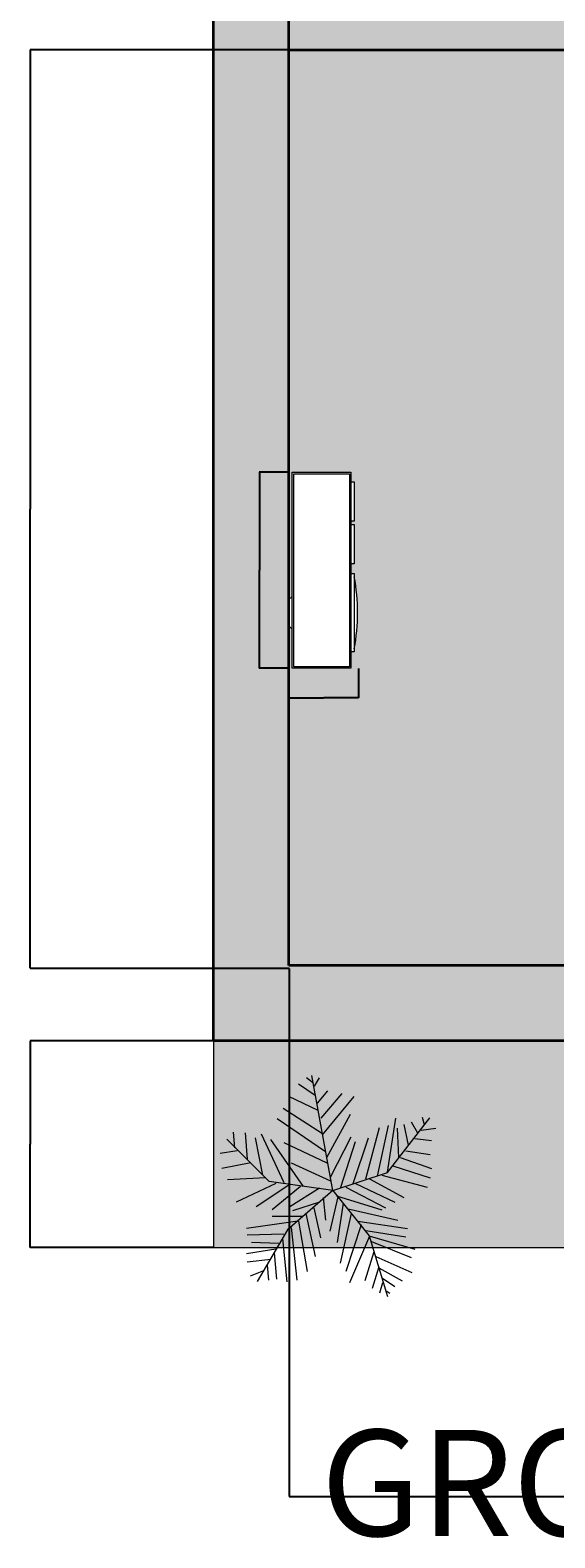
# Model space of a CAD drawing. Units: millimetres. Extents: x 1166 to 16630, y -7192 to 2820.
# Tile 1 of 8: x 1166 to 2769, y -7192 to -2583. Entities that reach past the tile are written whole.
import ezdxf

# ---------------------------------------------------------------- set-up
doc = ezdxf.new("R2010")
doc.units = ezdxf.units.MM
for name, color, linetype, lineweight in [('A-ANNO-DIMS', 2, 'Continuous', 18), ('A-ANNO-TEXT', 7, 'Continuous', 35), ('A-FURN', 8, 'Continuous', 18), ('A-WALL', 7, 'Continuous', 35), ('C-SITE-PAVE', 7, 'Continuous', 18), ('L-PLNT', 70, 'Continuous', 18), ('L-PLNT-PATT', 3, 'Continuous', 13)]:
    doc.layers.add(name, color=color, linetype=linetype, lineweight=lineweight)
doc.layers.add('A-FLOR-FNSH-PATT', color=254, linetype='Continuous', lineweight=13, true_color=0xfeeab9)
doc.layers.add('A-WALL-PATT', color=254, linetype='Continuous', lineweight=13, true_color=0xcecce6)
doc.styles.get("Standard").update_dxf_attribs({"font": 'arial.ttf'})
doc.dimstyles.get("Standard").update_dxf_attribs({"dimtxt": 0.18, "dimasz": 0.18, "dimexe": 0.18, "dimexo": 0.0625, "dimgap": 0.09, "dimtad": 0, "dimtih": 1, "dimtoh": 1, "dimdec": 4, "dimzin": 0, "dimdsep": 46, "dimtxsty": 'Standard', "dimcen": 0.09, "dimadec": 0, "dimazin": 0, "dimtfac": 1, "dimtdec": 4, "dimtofl": 0, "dimtmove": 0, "dimatfit": 3, "dimfxl": 1, "dimtolj": 1, "dimtzin": 0, "dimarcsym": 0})

# ---------------------------------------------------------------- blocks, each defined once
blk = doc.blocks.new('Entertainment Center')
for p, q in [((-4, 0), (-5, -1)), ((4, 0), (-4, 0)), ((5, -1), (4, 0)), ((-17, -19), (-17, -1)), ((-17, -1), (43, -1)), ((-16.5, -18.5), (-16.5, -1.5)), ((-16.5, -1.5), (42.5, -1.5)), ((42.5, -1.5), (42.5, -18.5)), ((43, -1), (43, -19)), ((43, -19), (-17, -19)), ((42.5, -18.5), (-16.5, -18.5)), ((-12, -20), (-12, -19)), ((12, -20), (-12, -20)), ((12, -19), (12, -20)), ((15, -20), (15, -19)), ((27, -20), (15, -20)), ((27, -19), (27, -20)), ((28, -20), (28, -19)), ((40, -20), (28, -20)), ((40, -19), (40, -20))]:
    blk.add_line(p, q)
blk.add_arc((0, 40), 61, 259.6111, 280.3889)
blk = doc.blocks.new('*U12')
for p, q in [((-8.737, 47.138), (-17.069, 52.711)), ((-10.186, 53.64), (-13.084, 55.962)), ((0, 0), (-10.5, 57)), ((-9.099, 51.782), (-6.563, 55.962)), ((-7.288, 39.707), (-21.778, 46.673)), ((-7.65, 43.423), (-2.578, 49.46)), ((-5.839, 35.992), (4.667, 48.067)), ((-5.114, 27.632), (10.463, 46.673)), ((-5.114, 28.097), (-24.676, 40.636)), ((-2.941, 16.486), (8.652, 37.85)), ((-3.665, 19.273), (-27.574, 35.527)), ((16.259, 5.805), (23.142, 31.348)), ((22.055, 7.198), (27.489, 32.277)), ((27, 9), (48, 36)), ((27.127, 9.056), (31.112, 35.992)), ((31.836, 30.883), (32.561, 16.486)), ((35.096, 32.741), (37.27, 22.524)), ((38.719, 34.134), (41.979, 28.561)), ((43.791, 29.954), (51.036, 30.883)), ((44.153, 36.456), (45.239, 32.741)), ((-31.5, 4.5), (-52.5, 25.5)), ((-48.585, 21.131), (-49.309, 29.026)), ((-43.513, 28.561), (-42.427, 15.558)), ((-38.442, 26.239), (-34.819, 7.663)), ((-35.544, 28.097), (-24.314, 3.947)), ((-14.533, 2.09), (-30.834, 25.31)), ((-24.314, 23.917), (-2.941, 13.7)), ((-1.129, 6.734), (9.014, 26.704)), ((3.942, 1.625), (11.187, 24.381)), ((10.101, 3.483), (17.708, 26.239)), ((40.53, 25.775), (48.862, 24.846)), ((-47.498, 19.737), (-55.83, 18.344)), ((33.285, 16.486), (48.862, 10.913)), ((36.183, 19.737), (48.137, 17.88)), ((-40.615, 13.7), (-55.105, 10.913)), ((-20.691, 13.7), (-1.129, 4.876)), ((0, 0), (27, 9)), ((24.229, 7.663), (46.688, 1.625)), ((29.662, 12.307), (48.137, 6.269)), ((-33.37, 6.269), (-52.207, 5.34)), ((-28.299, 3.483), (-47.86, -5.805)), ((-21.416, 3.018), (-38.079, -8.128)), ((0, 0), (-31.5, 4.5)), ((-15.982, 2.09), (-30.11, -9.521)), ((0, 0), (-22.5, -19.5)), ((-6.563, 1.161), (-21.416, -8.128)), ((0, 0), (18, -22.5)), ((6.478, 1.625), (26.04, -8.592)), ((11.187, 3.483), (30.749, -5.805)), ((18.07, 5.805), (35.096, -3.483)), ((-6.563, -5.805), (-19.967, -9.985)), ((-4.752, -3.483), (-3.665, -14.629)), ((2.493, -3.019), (-1.491, -20.202)), ((1.769, -2.555), (24.229, -9.521)), ((5.029, -6.27), (2.131, -25.775)), ((-15.257, -12.772), (-30.11, -12.772)), ((-13.446, -11.378), (-8.737, -32.741)), ((-9.461, -8.592), (-6.201, -23.453)), ((9.014, -11.378), (3.58, -35.992)), ((7.565, -9.056), (32.198, -14.629)), ((-17.431, -15.094), (-42.789, -18.809)), ((-24.314, -21.596), (-42.427, -22.06)), ((-22.5, -19.5), (-37.5, -45)), ((-20.691, -18.345), (-17.793, -44.352)), ((-17.069, -15.094), (-12.721, -40.172)), ((14.085, -16.951), (6.478, -40.172)), ((12.274, -15.094), (36.907, -18.809)), ((16.259, -19.738), (36.183, -22.989)), ((-28.299, -29.026), (-42.789, -31.348)), ((-26.849, -26.24), (-40.253, -25.775)), ((-25.038, -23.918), (-22.865, -45.281)), ((18.07, -22.524), (8.289, -45.745)), ((18, -22.5), (27, -52.5)), ((18.433, -22.524), (40.53, -29.026)), ((19.157, -25.311), (38.719, -33.206)), ((-30.834, -34.135), (-42.427, -35.528)), ((-32.646, -36.921), (-31.921, -44.352)), ((-29.023, -30.884), (-27.936, -43.887)), ((20.244, -30.419), (15.897, -44.816)), ((21.331, -32.741), (39.081, -40.636)), ((-34.457, -39.708), (-40.978, -42.494)), ((22.78, -37.85), (19.519, -48.532)), ((22.78, -38.314), (34.372, -44.816)), ((24.591, -43.423), (30.749, -47.603)), ((24.591, -45.745), (23.142, -50.854)), ((26.764, -49.925), (28.213, -50.854))]:
    blk.add_line(p, q)
blk = doc.blocks.new('*D17')
at = {"layer": 'A-ANNO-DIMS', "color": 0, "lineweight": -2, "transparency": 16777216}
for p, q in [((1955.9, -3933.8), (1865.8, -3933.8)), ((1866, -3934), (1866, -4233.5)), ((1866, -4533.4), (1866, -4233.8)), ((1955.9, -4533.5), (1865.8, -4533.5))]:
    blk.add_line(p, q, dxfattribs=at)
at = {"layer": 'A-ANNO-DIMS', "color": 0, "transparency": 16777216}
for points in [[(1865.9, -3934), (1866, -3934), (1866, -3933.8)], [(1865.9, -4533.4), (1866, -4533.4), (1866, -4533.5)]]:
    blk.add_solid(points, dxfattribs=at)
at = {"layer": 'Defpoints', "color": 0, "transparency": 16777216}
for p in [(1866, -3933.8), (1955.9, -3933.8), (1955.9, -4533.5)]:
    blk.add_point(p, dxfattribs=at)
at = {"layer": 'A-ANNO-DIMS', "color": 0, "transparency": 16777216, "insert": (1866, -4233.7), "char_height": 0.18, "attachment_point": 5}
blk.add_mtext('\\A1;TV UNIT 600 TYP.', dxfattribs=at)
blk = doc.blocks.new('*D18')
at = {"layer": 'A-ANNO-DIMS', "color": 0, "lineweight": -2, "transparency": 16777216}
for p, q in [((1955.9, -4533.6), (1955.9, -4623.7)), ((2169.2, -4533.6), (2169.2, -4623.7)), ((1956.1, -4623.5), (2062, -4623.5)), ((2169, -4623.5), (2063.2, -4623.5))]:
    blk.add_line(p, q, dxfattribs=at)
at = {"layer": 'A-ANNO-DIMS', "color": 0, "transparency": 16777216}
for points in [[(1956.1, -4623.5), (1956.1, -4623.5), (1955.9, -4623.5)], [(2169, -4623.5), (2169, -4623.5), (2169.2, -4623.5)]]:
    blk.add_solid(points, dxfattribs=at)
at = {"layer": 'Defpoints', "color": 0, "transparency": 16777216}
for p in [(1955.9, -4533.5), (2169.2, -4533.5), (1955.9, -4623.5)]:
    blk.add_point(p, dxfattribs=at)
at = {"layer": 'A-ANNO-DIMS', "color": 0, "transparency": 16777216, "insert": (2062.6, -4623.5), "char_height": 0.18, "attachment_point": 5}
blk.add_mtext('\\A1;213 TYP.', dxfattribs=at)
blk = doc.blocks.new('*D30')
at = {"layer": 'A-ANNO-DIMS', "color": 0, "lineweight": -2, "transparency": 16777216}
for p, q in [((1955.9, -2642.5), (1165.9, -2642.5)), ((1166.1, -2642.7), (1166.1, -4046.5)), ((1166.1, -5450.7), (1166.1, -4046.9)), ((1956.9, -5450.8), (1165.9, -5450.8))]:
    blk.add_line(p, q, dxfattribs=at)
at = {"layer": 'A-ANNO-DIMS', "color": 0, "transparency": 16777216}
for points in [[(1166.1, -2642.7), (1166.1, -2642.7), (1166.1, -2642.5)], [(1166.1, -5450.7), (1166.1, -5450.7), (1166.1, -5450.8)]]:
    blk.add_solid(points, dxfattribs=at)
at = {"layer": 'Defpoints', "color": 0, "transparency": 16777216}
for p in [(1955.9, -2642.5), (1166.1, -5450.8), (1957, -5450.8)]:
    blk.add_point(p, dxfattribs=at)
at = {"layer": 'A-ANNO-DIMS', "color": 0, "transparency": 16777216, "insert": (1166.1, -4046.7), "char_height": 0.18, "attachment_point": 5}
blk.add_mtext('\\A1;2808.3', dxfattribs=at)
blk = doc.blocks.new('*D31')
at = {"layer": 'A-ANNO-DIMS', "color": 0, "lineweight": -2, "transparency": 16777216}
for p, q in [((1957, -5450.9), (1957, -7065.6)), ((5189.6, -5442.6), (5189.6, -7065.6)), ((1957.2, -7065.4), (3572.8, -7065.4)), ((5189.4, -7065.4), (3573.8, -7065.4))]:
    blk.add_line(p, q, dxfattribs=at)
at = {"layer": 'A-ANNO-DIMS', "color": 0, "transparency": 16777216}
for points in [[(1957.2, -7065.4), (1957.2, -7065.5), (1957, -7065.4)], [(5189.4, -7065.4), (5189.4, -7065.5), (5189.6, -7065.4)]]:
    blk.add_solid(points, dxfattribs=at)
at = {"layer": 'Defpoints', "color": 0, "transparency": 16777216}
for p in [(1957, -5450.8), (5189.6, -5442.5), (5189.6, -7065.4)]:
    blk.add_point(p, dxfattribs=at)
at = {"layer": 'A-ANNO-DIMS', "color": 0, "transparency": 16777216, "insert": (3573.3, -7065.4), "char_height": 0.18, "attachment_point": 5}
blk.add_mtext('\\A1;3232.6', dxfattribs=at)
blk = doc.blocks.new('*D38')
at = {"layer": 'A-ANNO-DIMS', "color": 0, "lineweight": -2, "transparency": 16777216}
for p, q in [((1725.9, -5672.5), (1165.9, -5672.5)), ((1166.1, -5672.7), (1166.1, -5988.2)), ((1166.1, -6304), (1166.1, -5988.5)), ((1725.9, -6304.1), (1165.9, -6304.1))]:
    blk.add_line(p, q, dxfattribs=at)
at = {"layer": 'A-ANNO-DIMS', "color": 0, "transparency": 16777216}
for points in [[(1166.1, -5672.7), (1166.1, -5672.7), (1166.1, -5672.5)], [(1166.1, -6304), (1166.1, -6304), (1166.1, -6304.1)]]:
    blk.add_solid(points, dxfattribs=at)
at = {"layer": 'Defpoints', "color": 0, "transparency": 16777216}
for p in [(1725.9, -5672.5), (1166.1, -6304.1), (1725.9, -6304.1)]:
    blk.add_point(p, dxfattribs=at)
at = {"layer": 'A-ANNO-DIMS', "color": 0, "transparency": 16777216, "insert": (1166.1, -5988.3), "char_height": 0.18, "attachment_point": 5}
blk.add_mtext('\\A1;631.6', dxfattribs=at)

msp = doc.modelspace()

# ---------------------------------------------------------------- hatches: boundary and pattern name
at = {"layer": 'A-FLOR-FNSH-PATT', "transparency": 33554523}
h = msp.add_hatch(color=256, dxfattribs=at)
h.dxf.hatch_style = 1
h.paths.add_polyline_path([(7725.939, 2327.462), (1725.939, 2327.462), (1725.939, -5672.538), (5309.615, -5672.538), (5309.615, -2642.538), (5189.615, -2642.538), (5189.615, -5442.538), (1955.939, -5442.538), (1955.939, 2097.462), (4665.939, 2097.462), (4665.939, 150.2), (4815.939, 150.2, -0.40145271), (5814.982, -806.05), (5815.939, -806.05), (5815.939, -849.8), (4815.939, -849.8), (4785.939, -849.8), (4785.939, -902.538), (7495.939, -902.538), (7495.939, -2522.538), (4884.014, -2522.538), (4884.014, -2642.538), (7725.939, -2642.538)], flags=17)
h.paths.add_polyline_path([(6066.077, 618.421), (6066.077, 1624.186), (7407.098, 1624.186), (7407.098, 618.421)], flags=16)
h.paths.add_polyline_path([(4979.212, 660.219), (4799.278, 660.219), (4799.278, 780.174), (4789.282, 790.171), (4789.282, 870.141), (4799.278, 880.137), (4799.278, 1259.997), (4979.212, 1259.997), (4979.212, 1230.008), (4989.208, 1230.008), (4989.208, 1110.052), (4979.212, 1110.052), (4979.212, 1100.056), (4989.208, 1100.056), (4989.208, 980.1), (4979.212, 980.1), (4979.212, 950.111), (4989.208, 950.111), (4989.208, 940.115, -0.09090909), (4989.208, 720.196), (4989.208, 710.2), (4979.212, 710.2)], flags=16)
h.paths.add_polyline_path([(4974.214, 665.217), (4804.276, 665.217), (4804.276, 1254.999), (4974.214, 1254.999)], flags=0)
h.paths.add_polyline_path([(6910.92, 618.421), (6910.92, 873.215), (7165.714, 873.215), (7165.714, 1490.084), (7386.983, 1490.084), (7386.983, 1141.419), (7165.714, 1141.419), (7165.714, 1101.188), (7386.983, 1101.188), (7386.983, 752.523), (7132.189, 752.523), (7132.189, 839.689)], flags=16)
h.paths.add_polyline_path([(4815.939, 150.2), (4665.939, 150.2), (4665.939, 1500.697), (2460.545, 1500.697), (2460.545, -402.538), (3575.939, -402.538), (3575.939, -1706.64), (3463.439, -1706.64, 0.40145271), (2714.158, -2423.828), (3463.439, -2423.828), (3463.439, -2456.64), (3455.939, -2522.538), (3455.939, -2456.64), (2713.439, -2456.64), (2713.439, -2423.828), (2714.158, -2423.828, -0.39855266), (3455.939, -1706.678), (3455.939, -1706.64), (3575.939, -1706.64), (3575.939, -402.538), (2460.545, -402.538), (2460.545, 1500.697), (4665.939, 1500.697), (4665.939, 150.2), (4785.939, 150.2), (4785.939, 2097.462), (7495.939, 2097.462), (7495.939, -2522.538), (4884.014, -2522.538), (4884.014, -2642.538), (7725.939, -2642.538), (7725.939, 2327.462), (1725.939, 2327.462), (1725.939, -5672.538), (5309.615, -5672.538), (5309.615, -2642.538), (4884.014, -2642.538), (4884.014, -2522.538), (4884.014, -1822.538), (4665.939, -1822.538), (4665.939, -1722.538), (4665.939, -1022.538), (4665.939, -849.8), (4815.939, -849.8), (4815.939, -806.05), (5814.982, -806.05, 0.40145271)])
h.paths.add_polyline_path([(1955.939, -4323.626), (1965.936, -4313.63), (1965.936, -3933.77), (2145.869, -3933.77), (2145.869, -3963.759), (2155.866, -3963.759), (2155.866, -4083.715), (2145.869, -4083.715), (2145.869, -4093.711), (2155.866, -4093.711), (2155.866, -4213.667), (2145.869, -4213.667), (2145.869, -4243.656), (2155.866, -4243.656), (2155.866, -4253.652, -0.09090909), (2155.866, -4473.571), (2155.866, -4483.567), (2145.869, -4483.567), (2145.869, -4533.549), (1965.936, -4533.549), (1965.936, -4413.593), (1955.939, -4403.597)], flags=16)
h.paths.add_polyline_path([(3017.672, -1268.685), (3017.672, -1558.932), (2092.538, -1558.932), (2092.538, -1268.685)], flags=16)
h.paths.add_polyline_path([(2768.799, -687.028), (2664.904, -687.028), (2696.871, -782.93, -0.50132349), (2617.667, -1084.405, -0.13289091), (2584.271, -1084.405, -0.50131678), (2505.065, -782.933), (2537.033, -687.028), (2489.082, -687.028), (2489.082, -711.004), (2441.13, -711.004), (2441.13, -687.028), (2433.138, -687.028), (2433.138, -559.158), (2768.799, -559.158)], flags=16)
h.paths.add_polyline_path([(2752.815, -655.061, -0.41421356), (2740.827, -671.045), (2465.106, -671.045, -0.41421356), (2449.122, -659.057), (2449.122, -591.126, -0.41421356), (2461.11, -575.142), (2736.831, -575.142, -0.41421356), (2752.815, -587.13)], flags=0)
h.paths.add_polyline_path([(2627.247, -1063.016, -0.21500378), (2574.691, -1063.016, -0.48007965), (2537.034, -782.931), (2664.904, -782.931, -0.4800795)], flags=0)
h.paths.add_polyline_path([(4505.634, -3647.875), (4977.863, -3647.875, -0.19047621), (4977.864, -5173.541), (4505.634, -5173.541), (4505.634, -5064.565), (4533.929, -5064.565), (4533.929, -3756.851), (4505.634, -3756.851)], flags=16)
h.paths.add_polyline_path([(4880.114, -4192.756), (5003.372, -4192.756, -0.04962821), (5003.372, -4628.66), (4880.114, -4628.66)], flags=0)
h.paths.add_polyline_path([(2140.871, -3938.769), (2140.871, -4528.551), (1970.934, -4528.551), (1970.934, -3938.769)], flags=0)
h.paths.add_polyline_path([(7495.939, -1022.538), (6660.699, -1022.538), (6660.699, -1722.538, -0.21291191), (6697.901, -1739.132)], flags=16)
h.paths.add_polyline_path([(7495.939, -1022.538), (6697.901, -1739.132, -0.18498743), (6710.699, -1772.538), (7495.939, -1772.538)], flags=16)
h.paths.add_polyline_path([(7495.939, -1772.538), (6710.699, -1772.538, -0.18498743), (6697.901, -1805.944), (7495.939, -2522.538)], flags=16)
h.paths.add_polyline_path([(6697.901, -1805.944, -0.21291191), (6660.699, -1822.538), (6660.699, -2522.538), (7495.939, -2522.538)], flags=16)
h.paths.add_polyline_path([(6660.699, -1822.538), (6438.613, -1822.538), (6438.613, -2522.538), (6660.699, -2522.538)], flags=16)
h.paths.add_polyline_path([(6438.613, -1822.538), (6216.528, -1822.538), (6216.528, -2522.538), (6438.613, -2522.538)], flags=16)
h.paths.add_polyline_path([(6216.528, -1822.538), (5994.442, -1822.538), (5994.442, -2522.538), (6216.528, -2522.538)], flags=16)
h.paths.add_polyline_path([(5994.442, -1822.538), (5772.357, -1822.538), (5772.357, -2522.538), (5994.442, -2522.538)], flags=16)
h.paths.add_polyline_path([(5550.271, -1822.538), (5328.185, -1822.538), (5328.185, -2522.538), (5550.271, -2522.538)], flags=16)
h.paths.add_polyline_path([(5328.185, -1822.538), (5106.1, -1822.538), (5106.1, -2522.538), (5328.185, -2522.538)], flags=16)
h.paths.add_polyline_path([(5106.1, -1822.538), (4884.014, -1822.538), (4884.014, -2522.538), (5106.1, -2522.538)], flags=16)
h.paths.add_polyline_path([(4884.014, -1022.538), (4665.939, -1022.538), (4665.939, -1722.538), (4884.014, -1722.538)], flags=16)
h.paths.add_polyline_path([(5106.1, -1022.538), (4884.014, -1022.538), (4884.014, -1722.538), (5106.1, -1722.538)], flags=16)
h.paths.add_polyline_path([(5550.271, -1022.538), (5328.185, -1022.538), (5328.185, -1722.538), (5550.271, -1722.538)], flags=16)
h.paths.add_polyline_path([(5328.185, -1022.538), (5106.1, -1022.538), (5106.1, -1722.538), (5328.185, -1722.538)], flags=16)
h.paths.add_polyline_path([(5772.357, -1022.538), (5550.271, -1022.538), (5550.271, -1722.538), (5772.357, -1722.538)], flags=16)
h.paths.add_polyline_path([(5994.442, -1022.538), (5772.357, -1022.538), (5772.357, -1722.538), (5994.442, -1722.538)], flags=16)
h.paths.add_polyline_path([(6216.528, -1022.538), (5994.442, -1022.538), (5994.442, -1722.538), (6216.528, -1722.538)], flags=16)
h.paths.add_polyline_path([(6660.699, -1022.538), (6438.613, -1022.538), (6438.613, -1722.538), (6660.699, -1722.538)], flags=16)
h.paths.add_polyline_path([(6438.613, -1022.538), (6216.528, -1022.538), (6216.528, -1722.538), (6438.613, -1722.538)], flags=16)
h.paths.add_polyline_path([(5772.357, -1822.538), (5550.271, -1822.538), (5550.271, -2522.538), (5772.357, -2522.538)], flags=16)
h.paths.add_polyline_path([(6660.699, -1722.538), (6438.613, -1722.538), (4665.939, -1722.538), (4665.939, -1822.538), (6660.699, -1822.538, 0.21291191), (6697.901, -1805.944, 0.64892437)], flags=16)
h.paths.add_polyline_path([(5860.25, -44.006), (7154.504, -44.006), (7154.504, 215.689), (5860.25, 215.689)], flags=24)
h.paths.add_polyline_path([(2102.336, -1543.656), (3007.075, -1543.656), (3007.075, -1283.961), (2102.336, -1283.961)], flags=8)
h.paths.add_polyline_path([(2887.503, -4248.68), (3740.372, -4248.68), (3740.372, -3989.156), (2887.503, -3989.156)], flags=24)
h.paths.add_polyline_path([(2999.436, 433.054), (4111.829, 433.054), (4111.829, 692.578), (2999.436, 692.578)], flags=24)
at = {"layer": 'A-FLOR-FNSH-PATT', "transparency": 33554590}
h = msp.add_hatch(color=256, dxfattribs=at)
h.dxf.hatch_style = 1
h.paths.add_polyline_path([(5309.615, -2642.538), (5309.615, -6304.141), (7725.939, -6304.141), (7725.939, -5672.538), (7725.939, -2642.538)])
edge = h.paths.add_edge_path(flags=16)
edge.add_ellipse((-448.972, -3645.43), major_axis=(-7430.723, 0), ratio=0.84230387, start_angle=182.1799503, end_angle=183.6504276, ccw=False)
edge.add_line((6974.174, -3362.862), (6984.716, -3362.862))
edge.add_ellipse((6982.281, -3380.397), major_axis=(-20.817, 0), ratio=0.84230387, start_angle=180, end_angle=270, ccw=False)
edge.add_line((7003.098, -3380.397), (7003.098, -3722.916))
edge.add_ellipse((6982.281, -3720.865), major_axis=(20.817, 0), ratio=0.84230387, start_angle=270, end_angle=360, ccw=False)
edge.add_ellipse((-142030.923, -3973.064), major_axis=(149013.204, 0), ratio=0.8423038695, start_angle=-0.38386678, end_angle=0.09022909, ccw=False)
edge.add_line((6977.567, -4971.397), (6984.47, -4971.397))
edge.add_ellipse((6982.281, -4988.932), major_axis=(20.817, 0), ratio=0.84230387, start_angle=0, end_angle=90, ccw=False)
edge.add_line((7003.098, -4988.932), (7003.098, -5331.243))
edge.add_ellipse((6982.281, -5329.4), major_axis=(-20.817, 0), ratio=0.84230387, start_angle=90, end_angle=180, ccw=False)
edge.add_line((6982.281, -5346.934), (6973.354, -5346.934))
edge.add_ellipse((-142030.923, -3973.064), major_axis=(149013.204, 0), ratio=0.8423038695, start_angle=-0.6186432, end_angle=-0.52827147, ccw=False)
edge.add_ellipse((6960.189, -5606.903), major_axis=(-31.226, 0), ratio=0.84230387, start_angle=179.371763, end_angle=248.464757, ccw=False)
edge.add_ellipse((-142041.332, -3973.064), major_axis=(-149045.372, 0), ratio=0.8423038661, start_angle=179.35344592, end_angle=179.3717628, ccw=False)
edge.add_ellipse((6916.87, -5654.054), major_axis=(-73.802, 0), ratio=0.84230387, start_angle=90, end_angle=179.353446, ccw=False)
edge.add_line((6916.87, -5716.218), (5995.23, -5716.218))
edge.add_ellipse((5995.23, -5654.054), major_axis=(73.802, 0), ratio=0.84230387, start_angle=180.646554, end_angle=270, ccw=False)
edge.add_ellipse((154953.432, -3973.064), major_axis=(-149045.372, 0), ratio=0.8423038697, start_angle=0.62823722, end_angle=0.6465541, ccw=False)
edge.add_ellipse((5951.911, -5606.903), major_axis=(31.226, 0), ratio=0.84230387, start_angle=111.535244, end_angle=180.628237, ccw=False)
edge.add_ellipse((154943.023, -3973.064), major_axis=(-149013.204, 0), ratio=0.8423038695, start_angle=0.52827147, end_angle=0.6465541, ccw=False)
edge.add_line((5938.746, -5346.934), (5927.384, -5346.934))
edge.add_ellipse((5929.819, -5329.4), major_axis=(20.817, 0), ratio=0.84230387, start_angle=180, end_angle=270, ccw=False)
edge.add_line((5909.002, -5329.4), (5909.002, -4986.881))
edge.add_ellipse((5929.819, -4988.932), major_axis=(-20.817, 0), ratio=0.84230387, start_angle=-90, end_angle=0, ccw=False)
edge.add_line((5929.819, -4971.397), (5934.533, -4971.397))
edge.add_ellipse((154943.023, -3973.064), major_axis=(-149013.204, 0), ratio=0.8423038695, start_angle=-0.09022909, end_angle=0.38386678, ccw=False)
edge.add_ellipse((5929.819, -3720.865), major_axis=(-20.817, 0), ratio=0.84230387, start_angle=0, end_angle=90, ccw=False)
edge.add_line((5909.002, -3720.865), (5909.002, -3378.346))
edge.add_ellipse((5929.819, -3380.397), major_axis=(20.817, 0), ratio=0.84230387, start_angle=90, end_angle=180, ccw=False)
edge.add_line((5929.819, -3362.862), (5937.926, -3362.862))
edge.add_ellipse((13361.072, -3645.43), major_axis=(7430.723, 0), ratio=0.84230387, start_angle=176.3495724, end_angle=177.8200497, ccw=False)
edge.add_ellipse((6843.239, -6808.261), major_axis=(4407.333, 0), ratio=0.84230387, start_angle=102.125966, end_angle=103.780529, ccw=False)
edge.add_ellipse((6843.239, -6711.831), major_axis=(4294.728, 0), ratio=0.84230387, start_angle=100.209539, end_angle=102.444627, ccw=False)
edge.add_ellipse((5718.978, -189.342), major_axis=(-3530.283, 0), ratio=0.84230387, start_angle=99.256566, end_angle=102.554933)
edge.add_line((6369.843, -3111.939), (6452.047, -3066.483))
edge.add_ellipse((6456.05, -3074.757), major_axis=(-10.409, 0), ratio=0.84230387, start_angle=270, end_angle=307.93313, ccw=False)
edge.add_ellipse((6456.05, -3074.757), major_axis=(-10.409, 0), ratio=0.84230387, start_angle=232.06687, end_angle=270, ccw=False)
edge.add_line((6461.762, -3067.428), (6542.257, -3111.939))
edge.add_ellipse((7193.122, -189.342), major_axis=(3530.283, 0), ratio=0.84230387, start_angle=257.445067, end_angle=260.743434)
edge.add_ellipse((6068.861, -6711.831), major_axis=(4294.728, 0), ratio=0.84230387, start_angle=77.555373, end_angle=79.790461, ccw=False)
edge.add_ellipse((6068.861, -6808.261), major_axis=(-4407.333, 0), ratio=0.84230387, start_angle=256.219471, end_angle=257.874034, ccw=False)
edge = h.paths.add_edge_path(flags=0)
edge.add_ellipse((5799.636, -3484.806), major_axis=(790.133, 0), ratio=0.84230387, start_angle=0, end_angle=29.43857, ccw=False)
edge.add_line((6589.77, -3484.806), (6589.77, -3517.866))
edge.add_line((6589.77, -3517.866), (6615.397, -3517.866))
edge.add_ellipse((6612.95, -3526.633), major_axis=(10.409, 0), ratio=0.84230387, start_angle=45.519789, end_angle=90, ccw=False)
edge.add_line((6619.584, -3519.877), (6697.577, -3574.216))
edge.add_line((6697.577, -3574.216), (6697.577, -3782.552))
edge.add_ellipse((6643.673, -3780.461), major_axis=(5.016, 89.187), ratio=0.60383358, start_angle=106.342592, end_angle=270.997986, ccw=False)
edge.add_line((6589.77, -3793.028), (6589.77, -3484.806))
edge.add_ellipse((5799.636, -3484.806), major_axis=(790.133, 0), ratio=0.84230387, start_angle=0, end_angle=29.43857)
edge.add_ellipse((7112.464, -3484.806), major_axis=(-790.133, 0), ratio=0.84230387, start_angle=-29.43857, end_angle=0)
edge.add_line((6322.33, -3484.806), (6322.33, -3793.028))
edge.add_ellipse((6268.427, -3780.461), major_axis=(-5.016, 89.187), ratio=0.60383358, start_angle=89.002014, end_angle=253.657408, ccw=False)
edge.add_line((6214.523, -3782.552), (6214.523, -3574.216))
edge.add_line((6214.523, -3574.216), (6294.401, -3518.564))
edge.add_ellipse((6299.15, -3526.633), major_axis=(10.409, 0), ratio=0.84230387, start_angle=90, end_angle=134.480211, ccw=False)
edge.add_line((6299.15, -3517.866), (6322.33, -3517.866))
edge.add_line((6322.33, -3517.866), (6322.33, -3484.806))
edge.add_ellipse((7112.464, -3484.806), major_axis=(-790.133, 0), ratio=0.84230387, start_angle=-29.43857, end_angle=0, ccw=False)
edge = h.paths.add_edge_path(flags=0)
edge.add_line((6899.672, -4051.113), (6868.937, -4281.474))
edge.add_ellipse((6495.43, -5170.363), major_axis=(1119.455, 0), ratio=0.84230387, start_angle=67.208085, end_angle=85.12993)
edge.add_line((6575.565, -4229.86), (6336.535, -4229.86))
edge.add_ellipse((6416.67, -5170.363), major_axis=(1119.455, 0), ratio=0.84230387, start_angle=94.87007, end_angle=112.791915)
edge.add_line((6043.163, -4281.474), (6012.428, -4051.113))
edge.add_ellipse((6380.264, -4969.144), major_axis=(1150.303, 0), ratio=0.84230387, start_angle=94.277421, end_angle=111.834954, ccw=False)
edge.add_line((6307.939, -4002.156), (6604.161, -4002.156))
edge.add_ellipse((6531.836, -4969.144), major_axis=(-1150.303, 0), ratio=0.84230387, start_angle=248.165046, end_angle=265.722579, ccw=False)
edge = h.paths.add_edge_path(flags=0)
edge.add_ellipse((-142030.923, -3973.064), major_axis=(-148992.387, 0), ratio=0.8423038695, start_angle=179.62223581, end_angle=179.94440569, ccw=False)
edge.add_line((6956.9, -4955.389), (6903.068, -4744.03))
edge.add_ellipse((-45118.924, -4413.46), major_axis=(52023.473, 0), ratio=0.84230387, start_angle=-0.3640763, end_angle=0.1208974)
edge.add_line((6904.386, -4303.688), (6961.365, -4117.632))
edge = h.paths.add_edge_path(flags=0)
edge.add_line((5950.735, -4117.632), (6007.714, -4303.688))
edge.add_ellipse((58031.024, -4413.46), major_axis=(-52023.473, 0), ratio=0.84230387, start_angle=-0.1208974, end_angle=0.3640763)
edge.add_line((6009.031, -4744.03), (5955.2, -4955.389))
edge.add_ellipse((154943.023, -3973.064), major_axis=(-148992.387, 0), ratio=0.8423038696, start_angle=0.05559431, end_angle=0.37776419, ccw=False)
edge = h.paths.add_edge_path(flags=0)
edge.add_line((6868.937, -5013.198), (6868.937, -5277.993))
edge.add_ellipse((6456.05, -3571.079), major_axis=(2068.116, 0), ratio=0.84230387, start_angle=256.401865, end_angle=283.598135, ccw=False)
edge.add_line((6043.163, -5277.993), (6043.163, -5013.198))
edge.add_ellipse((6456.05, -3306.285), major_axis=(2068.116, 0), ratio=0.84230387, start_angle=256.401865, end_angle=283.598135)
edge = h.paths.add_edge_path(flags=0)
edge.add_ellipse((6827.303, -5415.313), major_axis=(-41.634, 0), ratio=0.84230387, start_angle=180, end_angle=270, ccw=False)
edge.add_line((6868.937, -5415.313), (6868.937, -5689.123))
edge.add_line((6868.937, -5689.123), (6043.163, -5689.123))
edge.add_line((6043.163, -5689.123), (6043.163, -5415.313))
edge.add_ellipse((6084.797, -5415.313), major_axis=(-41.634, 0), ratio=0.84230387, start_angle=-90, end_angle=0, ccw=False)
edge.add_line((6084.797, -5380.245), (6827.303, -5380.245))
h.paths.add_polyline_path([(3455.939, -522.538), (1955.939, -522.538), (1955.939, -2522.538), (3455.939, -2522.538), (3455.939, -2456.64), (2713.439, -2456.64), (2713.439, -2423.828), (2714.158, -2423.828, -0.39855266), (3455.939, -1706.678)])
h.paths.add_polyline_path([(2617.667, -1084.405, -0.13289091), (2584.271, -1084.405, -0.50131678), (2505.065, -782.933), (2537.033, -687.028), (2489.082, -687.028), (2489.082, -711.004), (2441.13, -711.004), (2441.13, -695.02), (2473.098, -695.02), (2473.098, -687.028), (2433.138, -687.028), (2433.138, -559.158), (2768.799, -559.158), (2768.799, -687.028), (2664.904, -687.028), (2696.871, -782.93, -0.50132349)], flags=16)
h.paths.add_polyline_path([(2627.247, -1063.016, -0.21500378), (2574.691, -1063.016, -0.48007965), (2537.034, -782.931), (2664.904, -782.931, -0.4800795)], flags=0)
h.paths.add_polyline_path([(2736.831, -671.045), (2465.106, -671.045, -0.50000012), (2449.122, -655.061), (2449.122, -591.126, -0.50000012), (2465.106, -575.142), (2736.831, -575.142, -0.50000012), (2752.815, -591.126), (2752.815, -655.061, -0.50000012)], flags=0)
h.paths.add_polyline_path([(5931.782, -6111.826), (7070.31, -6111.826), (7070.31, -5852.302), (5931.782, -5852.302)], flags=24)
h.paths.add_polyline_path([(2102.336, -1543.656), (3007.075, -1543.656), (3007.075, -1283.961), (2102.336, -1283.961)], flags=24)
at = {"layer": 'A-WALL-PATT'}
h = msp.add_hatch(color=256, dxfattribs=at)
h.dxf.hatch_style = 1
h.paths.add_polyline_path([(1955.939, 2097.462), (4665.939, 2097.462), (4665.939, 150.2), (4785.939, 150.2), (4785.939, 2097.462), (7495.939, 2097.462), (7495.939, -2522.538), (4884.014, -2522.538), (4884.014, -2642.538), (7725.939, -2642.538), (7725.939, 2327.462), (1725.939, 2327.462), (1725.939, -5672.538), (5309.615, -5672.538), (5309.615, -2642.538), (5189.615, -2642.538), (5189.615, -5442.538), (1955.939, -5442.538)])
h.paths.add_polyline_path([(7495.939, -902.538), (4785.939, -902.538), (4785.939, -849.8), (4665.939, -849.8), (4665.939, -1022.538), (7495.939, -1022.538)], flags=17)
h.paths.add_polyline_path([(3575.939, -402.538), (1955.939, -402.538), (1955.939, -522.538), (3455.939, -522.538), (3455.939, -1706.64), (3575.939, -1706.64)], flags=17)
h.paths.add_polyline_path([(3575.939, -2456.64), (3455.939, -2456.64), (3455.939, -2522.538), (1955.939, -2522.538), (1955.939, -2642.538), (3575.939, -2642.538)], flags=17)
at = {"layer": 'L-PLNT-PATT'}
h = msp.add_hatch(dxfattribs=at)
h.set_pattern_fill('CROSS', color=256, scale=5)
h.set_pattern_definition([(0, (-8657.52, -11987.852), (31.75, 31.75), [15.875, -47.625]), (90, (-8649.582, -11995.79), (-31.75, 31.75), [15.875, -47.625])])
h.paths.add_polyline_path([(5309.615, -5672.538), (1725.939, -5672.538), (1725.939, -6304.141), (5189.615, -6304.141), (5309.615, -6304.141)])

# ---------------------------------------------------------------- linework, layer by layer
at = {"layer": 'A-WALL'}
for p, q in [((1955.939, -5442.538), (1955.939, 2097.462)), ((1955.939, -2642.538), (3575.939, -2642.538)), ((5189.615, -5442.538), (1955.939, -5442.538))]:
    msp.add_line(p, q, dxfattribs=at)
msp.add_lwpolyline([(5309.615, -5672.538), (1725.939, -5672.538), (1725.939, 2327.462), (7725.939, 2327.462), (7725.939, -5672.538)], dxfattribs=at)
at = {"layer": 'C-SITE-PAVE'}
for p, q in [((1725.939, -5672.538), (1725.939, -6304.141)), ((1725.939, -6304.141), (5189.615, -6304.141))]:
    msp.add_line(p, q, dxfattribs=at)

# ---------------------------------------------------------------- block references
at = {"layer": 'A-FURN', "xscale": 9.996305784360949, "yscale": 9.996305784360949, "zscale": 9.996305784360949, "rotation": 89.99999999999999}
msp.add_blockref('Entertainment Center', (1955.939, -4363.612), dxfattribs=at)
at = {"layer": 'L-PLNT', "xscale": 6.165566864666302, "yscale": 6.165566864666302, "zscale": 6.165566864666302}
msp.add_blockref('*U12', (2090.578, -6130.225), dxfattribs=at)

# ---------------------------------------------------------------- texts
at = {"layer": 'A-ANNO-TEXT'}
msp.add_text('GROUND FLOOR PLAN', height=324.44434, dxfattribs=at).set_placement((2053.876, -7186.111))

# ---------------------------------------------------------------- dimensions: what is measured, and where the dimension line sits
at = {"layer": 'A-ANNO-DIMS'}
for base, p1, p2, picture, middle in [((1166.088, -5450.841), (1955.939, -2642.538), (1956.988, -5450.841), '*D30', (1166.088, -4046.69)), ((1166.088, -6304.141), (1725.939, -5672.538), (1725.939, -6304.141), '*D38', (1166.088, -5988.339))]:
    dim = msp.add_linear_dim(base=base, p1=p1, p2=p2, angle=90, dimstyle='Standard', override={"dimdec": 1, "dimlfac": 1, "dimrnd": 0, "dimzin": 0, "dimdsep": 46, "dimlunit": 2}, dxfattribs=at)
    dim.commit()
    dim.dimension.update_dxf_attribs({"geometry": picture, "text_midpoint": middle})
for base, p1, p2, angle, text, picture, middle in [((1865.973, -3933.77), (1955.939, -4533.549), (1955.939, -3933.77), 90, 'TV UNIT <> TYP.', '*D17', (1865.973, -4233.66)), ((1955.939, -4623.516), (2169.194, -4533.549), (1955.939, -4533.549), 180, '<> TYP.', '*D18', (2062.567, -4623.516))]:
    dim = msp.add_linear_dim(base=base, p1=p1, p2=p2, angle=angle, text=text, dimstyle='Standard', override={"dimdec": 0, "dimlfac": 1, "dimrnd": 0, "dimzin": 0, "dimdsep": 46, "dimlunit": 2}, dxfattribs=at)
    dim.commit()
    dim.dimension.update_dxf_attribs({"geometry": picture, "text_midpoint": middle})
dim = msp.add_linear_dim(base=(5189.615, -7065.449), p1=(1956.988, -5450.841), p2=(5189.615, -5442.538), dimstyle='Standard', override={"dimdec": 1, "dimlfac": 1, "dimrnd": 0, "dimzin": 0, "dimdsep": 46, "dimlunit": 2}, dxfattribs=at)
dim.commit()
dim.dimension.update_dxf_attribs({"geometry": '*D31', "text_midpoint": (3573.302, -7065.449)})

doc.saveas('drawing.dxf')
